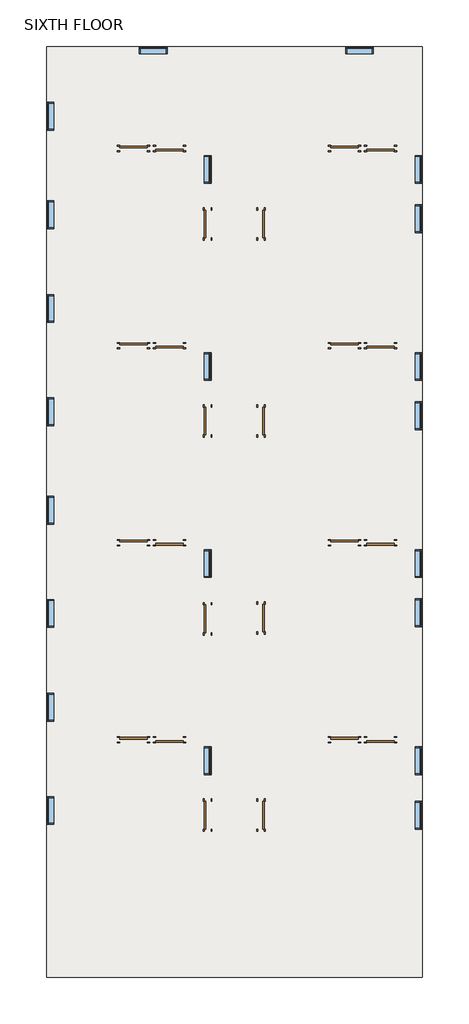
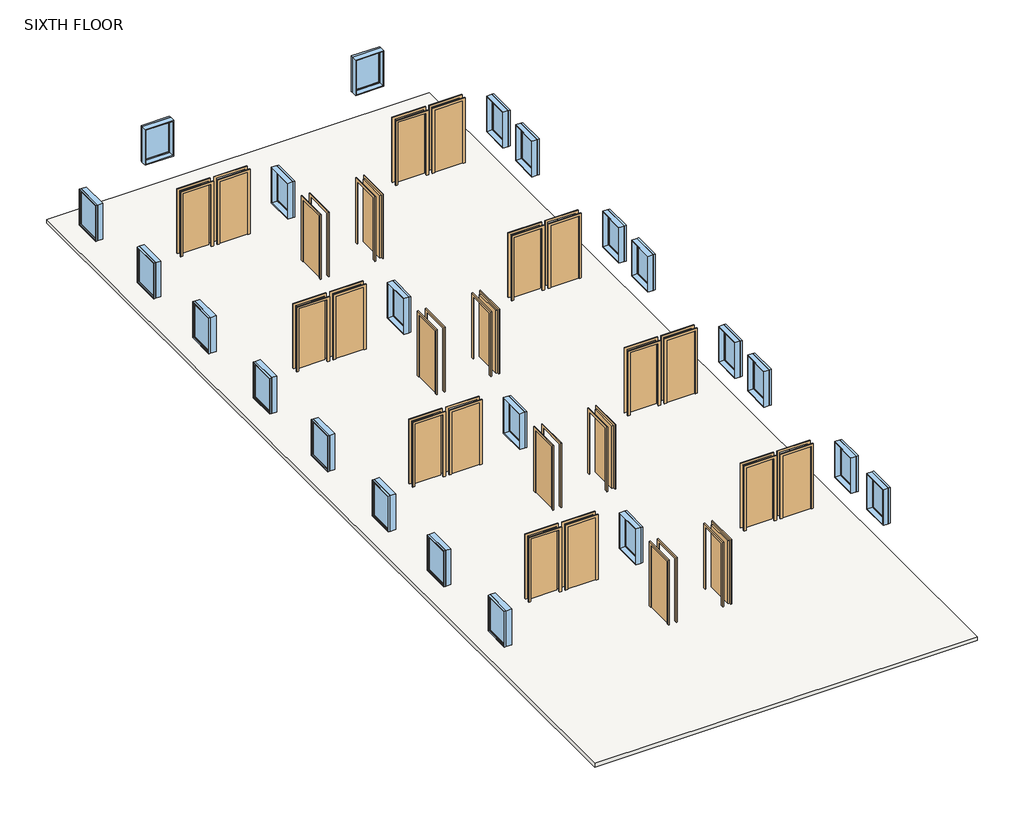
# One storey: 24 doors, 22 windows, 1 slab.
"""IFC4 building model written with IfcOpenShell, lengths in millimetres."""

from ifc_helpers import new_model, si_unit, frame, origin, place, context, project, spatial, polyline, outline, extrude, transform, mapped, element, save
from components import door_686f89d2, door_16372e1c, door_a90ba1ad, door_0ca8825f, window_c1f32544

model = new_model("IFC4")

# Units and contexts
model_context = context("Model", 3, world=origin())
ifc_project = project(units=[si_unit("LENGTHUNIT", "METRE", prefix="MILLI")], contexts=[model_context])

# Site, building, storey
site = spatial("IfcSite", under=ifc_project)
building = spatial("IfcBuilding", under=site)
storey = spatial("IfcBuildingStorey", under=building, Name="SIXTH FLOOR", Elevation=19202.4)

# Doors
placement = place(None, origin())
door_shape = door_686f89d2(model_context)
element("IfcDoor", 1, ObjectType="Single-Flush : 36\" x 84\"", at=placement, inside=storey, context=model_context, shape_type="MappedRepresentation", body=[
    mapped(door_shape, transform((-9863.5902461, 11952.2710592, 19202.4), x_axis=(-1.0, 0.0, 0.0), y_axis=(0.0, -1.0, 0.0), z_axis=(0.0, 0.0, 1.0))),
])
element("IfcDoor", 2, ObjectType="Single-Flush : 36\" x 84\"", at=placement, inside=storey, context=model_context, shape_type="MappedRepresentation", body=[
    mapped(door_shape, transform((-9863.5902461, 5475.2710592, 19202.4), x_axis=(-1.0, 0.0, 0.0), y_axis=(0.0, -1.0, 0.0), z_axis=(0.0, 0.0, 1.0))),
])
element("IfcDoor", 3, ObjectType="Single-Flush : 36\" x 84\"", at=placement, inside=storey, context=model_context, shape_type="MappedRepresentation", body=[
    mapped(door_shape, transform((-9863.5902461, -1001.7289408, 19202.4), x_axis=(-1.0, 0.0, 0.0), y_axis=(0.0, -1.0, 0.0), z_axis=(0.0, 0.0, 1.0))),
])
element("IfcDoor", 4, ObjectType="Single-Flush : 36\" x 84\"", at=placement, inside=storey, context=model_context, shape_type="MappedRepresentation", body=[
    mapped(door_shape, transform((-9863.5902461, -7478.7289408, 19202.4), x_axis=(-1.0, 0.0, 0.0), y_axis=(0.0, -1.0, 0.0), z_axis=(0.0, 0.0, 1.0))),
])
element("IfcDoor", 5, ObjectType="Single-Flush : 36\" x 84\"", at=placement, inside=storey, context=model_context, shape_type="MappedRepresentation", body=[
    mapped(door_shape, transform((-2929.3902461, -7478.7289408, 19202.4), x_axis=(-1.0, 0.0, 0.0), y_axis=(0.0, -1.0, 0.0), z_axis=(0.0, 0.0, 1.0))),
])
element("IfcDoor", 6, ObjectType="Single-Flush : 36\" x 84\"", at=placement, inside=storey, context=model_context, shape_type="MappedRepresentation", body=[
    mapped(door_shape, transform((-2929.3902461, -1001.7289408, 19202.4), x_axis=(-1.0, 0.0, 0.0), y_axis=(0.0, -1.0, 0.0), z_axis=(0.0, 0.0, 1.0))),
])
element("IfcDoor", 7, ObjectType="Single-Flush : 36\" x 84\"", at=placement, inside=storey, context=model_context, shape_type="MappedRepresentation", body=[
    mapped(door_shape, transform((-2929.3902461, 5475.2710592, 19202.4), x_axis=(-1.0, 0.0, 0.0), y_axis=(0.0, -1.0, 0.0), z_axis=(0.0, 0.0, 1.0))),
])
element("IfcDoor", 8, ObjectType="Single-Flush : 36\" x 84\"", at=placement, inside=storey, context=model_context, shape_type="MappedRepresentation", body=[
    mapped(door_shape, transform((-2929.3902461, 11952.2710592, 19202.4), x_axis=(-1.0, 0.0, 0.0), y_axis=(0.0, -1.0, 0.0), z_axis=(0.0, 0.0, 1.0))),
])
door_2_shape = door_16372e1c(model_context)
element("IfcDoor", 9, ObjectType="Single-Flush : 36\" x 84\"", at=placement, inside=storey, context=model_context, shape_type="MappedRepresentation", body=[
    mapped(door_2_shape, transform((-8682.4902461, 11952.2710592, 19202.4), x_axis=(-1.0, 0.0, 0.0), y_axis=(0.0, -1.0, 0.0), z_axis=(0.0, 0.0, 1.0))),
])
element("IfcDoor", 10, ObjectType="Single-Flush : 36\" x 84\"", at=placement, inside=storey, context=model_context, shape_type="MappedRepresentation", body=[
    mapped(door_2_shape, transform((-8682.4902461, 5475.2710592, 19202.4), x_axis=(-1.0, 0.0, 0.0), y_axis=(0.0, -1.0, 0.0), z_axis=(0.0, 0.0, 1.0))),
])
element("IfcDoor", 11, ObjectType="Single-Flush : 36\" x 84\"", at=placement, inside=storey, context=model_context, shape_type="MappedRepresentation", body=[
    mapped(door_2_shape, transform((-8682.4902461, -1001.7289408, 19202.4), x_axis=(-1.0, 0.0, 0.0), y_axis=(0.0, -1.0, 0.0), z_axis=(0.0, 0.0, 1.0))),
])
element("IfcDoor", 12, ObjectType="Single-Flush : 36\" x 84\"", at=placement, inside=storey, context=model_context, shape_type="MappedRepresentation", body=[
    mapped(door_2_shape, transform((-8682.4902461, -7478.7289408, 19202.4), x_axis=(-1.0, 0.0, 0.0), y_axis=(0.0, -1.0, 0.0), z_axis=(0.0, 0.0, 1.0))),
])
element("IfcDoor", 13, ObjectType="Single-Flush : 36\" x 84\"", at=placement, inside=storey, context=model_context, shape_type="MappedRepresentation", body=[
    mapped(door_2_shape, transform((-1748.2902461, -7478.7289408, 19202.4), x_axis=(-1.0, 0.0, 0.0), y_axis=(0.0, -1.0, 0.0), z_axis=(0.0, 0.0, 1.0))),
])
element("IfcDoor", 14, ObjectType="Single-Flush : 36\" x 84\"", at=placement, inside=storey, context=model_context, shape_type="MappedRepresentation", body=[
    mapped(door_2_shape, transform((-1748.2902461, -1001.7289408, 19202.4), x_axis=(-1.0, 0.0, 0.0), y_axis=(0.0, -1.0, 0.0), z_axis=(0.0, 0.0, 1.0))),
])
element("IfcDoor", 15, ObjectType="Single-Flush : 36\" x 84\"", at=placement, inside=storey, context=model_context, shape_type="MappedRepresentation", body=[
    mapped(door_2_shape, transform((-1748.2902461, 5475.2710592, 19202.4), x_axis=(-1.0, 0.0, 0.0), y_axis=(0.0, -1.0, 0.0), z_axis=(0.0, 0.0, 1.0))),
])
element("IfcDoor", 16, ObjectType="Single-Flush : 36\" x 84\"", at=placement, inside=storey, context=model_context, shape_type="MappedRepresentation", body=[
    mapped(door_2_shape, transform((-1748.2902461, 11952.2710592, 19202.4), x_axis=(-1.0, 0.0, 0.0), y_axis=(0.0, -1.0, 0.0), z_axis=(0.0, 0.0, 1.0))),
])
door_3_shape = door_a90ba1ad(model_context)
element("IfcDoor", 17, ObjectType="Single-Flush : 36\" x 84\"", at=placement, inside=storey, context=model_context, shape_type="MappedRepresentation", body=[
    mapped(door_3_shape, transform((-7425.1902461, 9475.7710592, 19202.4), x_axis=(0.0, -1.0, 0.0), y_axis=(1.0, 0.0, 0.0), z_axis=(0.0, 0.0, 1.0))),
])
element("IfcDoor", 18, ObjectType="Single-Flush : 36\" x 84\"", at=placement, inside=storey, context=model_context, shape_type="MappedRepresentation", body=[
    mapped(door_3_shape, transform((-7425.1902461, 2998.7710592, 19202.4), x_axis=(0.0, -1.0, 0.0), y_axis=(1.0, 0.0, 0.0), z_axis=(0.0, 0.0, 1.0))),
])
element("IfcDoor", 19, ObjectType="Single-Flush : 36\" x 84\"", at=placement, inside=storey, context=model_context, shape_type="MappedRepresentation", body=[
    mapped(door_3_shape, transform((-7425.1902461, -3503.6289408, 19202.4), x_axis=(0.0, -1.0, 0.0), y_axis=(1.0, 0.0, 0.0), z_axis=(0.0, 0.0, 1.0))),
])
element("IfcDoor", 20, ObjectType="Single-Flush : 36\" x 84\"", at=placement, inside=storey, context=model_context, shape_type="MappedRepresentation", body=[
    mapped(door_3_shape, transform((-7425.1902461, -9955.2289408, 19202.4), x_axis=(0.0, -1.0, 0.0), y_axis=(1.0, 0.0, 0.0), z_axis=(0.0, 0.0, 1.0))),
])
door_4_shape = door_0ca8825f(model_context)
element("IfcDoor", 21, ObjectType="Single-Flush : 36\" x 84\"", at=placement, inside=storey, context=model_context, shape_type="MappedRepresentation", body=[
    mapped(door_4_shape, transform((-5672.5902461, 9475.7710592, 19202.4), x_axis=(0.0, -1.0, 0.0), y_axis=(1.0, 0.0, 0.0), z_axis=(0.0, 0.0, 1.0))),
])
element("IfcDoor", 22, ObjectType="Single-Flush : 36\" x 84\"", at=placement, inside=storey, context=model_context, shape_type="MappedRepresentation", body=[
    mapped(door_4_shape, transform((-5672.5902461, 2998.7710592, 19202.4), x_axis=(0.0, -1.0, 0.0), y_axis=(1.0, 0.0, 0.0), z_axis=(0.0, 0.0, 1.0))),
])
element("IfcDoor", 23, ObjectType="Single-Flush : 36\" x 84\"", at=placement, inside=storey, context=model_context, shape_type="MappedRepresentation", body=[
    mapped(door_4_shape, transform((-5672.5902461, -3478.2289408, 19202.4), x_axis=(0.0, -1.0, 0.0), y_axis=(1.0, 0.0, 0.0), z_axis=(0.0, 0.0, 1.0))),
])
element("IfcDoor", 24, ObjectType="Single-Flush : 36\" x 84\"", at=placement, inside=storey, context=model_context, shape_type="MappedRepresentation", body=[
    mapped(door_4_shape, transform((-5672.5902461, -9955.2289408, 19202.4), x_axis=(0.0, -1.0, 0.0), y_axis=(1.0, 0.0, 0.0), z_axis=(0.0, 0.0, 1.0))),
])

# Slab
element("IfcSlab", 25, ObjectType="Generic - 12\"", at=placement, inside=storey, context=model_context, shape_type="SweptSolid", body=[
    extrude(outline(polyline([(-376.6902461, 15305.0710592), (-376.6902461, -15289.2289408), (-12721.0902461, -15289.2289408), (-12721.0902461, 15305.0710592), (-376.6902461, 15305.0710592)])), frame((0.0, 0.0, 19075.4), z_axis=(0.0, 0.0, 1.0), x_axis=(1.0, 0.0, 0.0)), (0.0, 0.0, 1.0), 127.0),
])

# Windows
window_shape = window_c1f32544(model_context)
element("IfcWindow", 26, ObjectType="Fixed : 36\" x 48\"", at=placement, inside=storey, context=model_context, shape_type="MappedRepresentation", body=[
    mapped(window_shape, transform((-9177.7902461, 15190.7710592, 19202.4), x_axis=(1.0, 0.0, 0.0), y_axis=(0.0, 1.0, 0.0), z_axis=(0.0, 0.0, 1.0))),
])
element("IfcWindow", 27, ObjectType="Fixed : 36\" x 48\"", at=placement, inside=storey, context=model_context, shape_type="MappedRepresentation", body=[
    mapped(window_shape, transform((-2395.9902461, 15190.7710592, 19202.4), x_axis=(1.0, 0.0, 0.0), y_axis=(0.0, 1.0, 0.0), z_axis=(0.0, 0.0, 1.0))),
])
element("IfcWindow", 28, ObjectType="Fixed : 36\" x 48\"", at=placement, inside=storey, context=model_context, shape_type="MappedRepresentation", body=[
    mapped(window_shape, transform((-490.9902461, 11228.3710592, 19202.4), x_axis=(0.0, -1.0, 0.0), y_axis=(1.0, 0.0, 0.0), z_axis=(0.0, 0.0, 1.0))),
])
element("IfcWindow", 29, ObjectType="Fixed : 36\" x 48\"", at=placement, inside=storey, context=model_context, shape_type="MappedRepresentation", body=[
    mapped(window_shape, transform((-490.9902461, 9609.1210592, 19202.4), x_axis=(0.0, -1.0, 0.0), y_axis=(1.0, 0.0, 0.0), z_axis=(0.0, 0.0, 1.0))),
])
element("IfcWindow", 30, ObjectType="Fixed : 36\" x 48\"", at=placement, inside=storey, context=model_context, shape_type="MappedRepresentation", body=[
    mapped(window_shape, transform((-490.9902461, 4751.3710592, 19202.4), x_axis=(0.0, -1.0, 0.0), y_axis=(1.0, 0.0, 0.0), z_axis=(0.0, 0.0, 1.0))),
])
element("IfcWindow", 31, ObjectType="Fixed : 36\" x 48\"", at=placement, inside=storey, context=model_context, shape_type="MappedRepresentation", body=[
    mapped(window_shape, transform((-490.9902461, 3132.1210592, 19202.4), x_axis=(0.0, -1.0, 0.0), y_axis=(1.0, 0.0, 0.0), z_axis=(0.0, 0.0, 1.0))),
])
element("IfcWindow", 32, ObjectType="Fixed : 36\" x 48\"", at=placement, inside=storey, context=model_context, shape_type="MappedRepresentation", body=[
    mapped(window_shape, transform((-490.9902461, -1725.6289408, 19202.4), x_axis=(0.0, -1.0, 0.0), y_axis=(1.0, 0.0, 0.0), z_axis=(0.0, 0.0, 1.0))),
])
element("IfcWindow", 33, ObjectType="Fixed : 36\" x 48\"", at=placement, inside=storey, context=model_context, shape_type="MappedRepresentation", body=[
    mapped(window_shape, transform((-490.9902461, -3344.8789408, 19202.4), x_axis=(0.0, -1.0, 0.0), y_axis=(1.0, 0.0, 0.0), z_axis=(0.0, 0.0, 1.0))),
])
element("IfcWindow", 34, ObjectType="Fixed : 36\" x 48\"", at=placement, inside=storey, context=model_context, shape_type="MappedRepresentation", body=[
    mapped(window_shape, transform((-490.9902461, -8202.6289408, 19202.4), x_axis=(0.0, -1.0, 0.0), y_axis=(1.0, 0.0, 0.0), z_axis=(0.0, 0.0, 1.0))),
])
element("IfcWindow", 35, ObjectType="Fixed : 36\" x 48\"", at=placement, inside=storey, context=model_context, shape_type="MappedRepresentation", body=[
    mapped(window_shape, transform((-490.9902461, -9993.3289408, 19202.4), x_axis=(0.0, -1.0, 0.0), y_axis=(1.0, 0.0, 0.0), z_axis=(0.0, 0.0, 1.0))),
])
element("IfcWindow", 36, ObjectType="Fixed : 36\" x 48\"", at=placement, inside=storey, context=model_context, shape_type="MappedRepresentation", body=[
    mapped(window_shape, transform((-12606.7902461, -9764.7289408, 19202.4), x_axis=(0.0, 1.0, 0.0), y_axis=(-1.0, 0.0, 0.0), z_axis=(0.0, 0.0, 1.0))),
])
element("IfcWindow", 37, ObjectType="Fixed : 36\" x 48\"", at=placement, inside=storey, context=model_context, shape_type="MappedRepresentation", body=[
    mapped(window_shape, transform((-12606.7902461, -6373.8289408, 19202.4), x_axis=(0.0, 1.0, 0.0), y_axis=(-1.0, 0.0, 0.0), z_axis=(0.0, 0.0, 1.0))),
])
element("IfcWindow", 38, ObjectType="Fixed : 36\" x 48\"", at=placement, inside=storey, context=model_context, shape_type="MappedRepresentation", body=[
    mapped(window_shape, transform((-12606.7902461, -3287.7289408, 19202.4), x_axis=(0.0, 1.0, 0.0), y_axis=(-1.0, 0.0, 0.0), z_axis=(0.0, 0.0, 1.0))),
])
element("IfcWindow", 39, ObjectType="Fixed : 36\" x 48\"", at=placement, inside=storey, context=model_context, shape_type="MappedRepresentation", body=[
    mapped(window_shape, transform((-12606.7902461, 103.1710592, 19202.4), x_axis=(0.0, 1.0, 0.0), y_axis=(-1.0, 0.0, 0.0), z_axis=(0.0, 0.0, 1.0))),
])
element("IfcWindow", 40, ObjectType="Fixed : 36\" x 48\"", at=placement, inside=storey, context=model_context, shape_type="MappedRepresentation", body=[
    mapped(window_shape, transform((-12606.7902461, 3341.6710592, 19202.4), x_axis=(0.0, 1.0, 0.0), y_axis=(-1.0, 0.0, 0.0), z_axis=(0.0, 0.0, 1.0))),
])
element("IfcWindow", 41, ObjectType="Fixed : 36\" x 48\"", at=placement, inside=storey, context=model_context, shape_type="MappedRepresentation", body=[
    mapped(window_shape, transform((-12606.7902461, 6732.5710592, 19202.4), x_axis=(0.0, 1.0, 0.0), y_axis=(-1.0, 0.0, 0.0), z_axis=(0.0, 0.0, 1.0))),
])
element("IfcWindow", 42, ObjectType="Fixed : 36\" x 48\"", at=placement, inside=storey, context=model_context, shape_type="MappedRepresentation", body=[
    mapped(window_shape, transform((-12606.7902461, 9818.6710592, 19202.4), x_axis=(0.0, 1.0, 0.0), y_axis=(-1.0, 0.0, 0.0), z_axis=(0.0, 0.0, 1.0))),
])
element("IfcWindow", 43, ObjectType="Fixed : 36\" x 48\"", at=placement, inside=storey, context=model_context, shape_type="MappedRepresentation", body=[
    mapped(window_shape, transform((-12606.7902461, 13057.1710592, 19202.4), x_axis=(0.0, 1.0, 0.0), y_axis=(-1.0, 0.0, 0.0), z_axis=(0.0, 0.0, 1.0))),
])
element("IfcWindow", 44, ObjectType="Fixed : 36\" x 48\"", at=placement, inside=storey, context=model_context, shape_type="MappedRepresentation", body=[
    mapped(window_shape, transform((-7425.1902461, 11228.3710592, 19202.4), x_axis=(0.0, -1.0, 0.0), y_axis=(1.0, 0.0, 0.0), z_axis=(0.0, 0.0, 1.0))),
])
element("IfcWindow", 45, ObjectType="Fixed : 36\" x 48\"", at=placement, inside=storey, context=model_context, shape_type="MappedRepresentation", body=[
    mapped(window_shape, transform((-7425.1902461, 4751.3710592, 19202.4), x_axis=(0.0, -1.0, 0.0), y_axis=(1.0, 0.0, 0.0), z_axis=(0.0, 0.0, 1.0))),
])
element("IfcWindow", 46, ObjectType="Fixed : 36\" x 48\"", at=placement, inside=storey, context=model_context, shape_type="MappedRepresentation", body=[
    mapped(window_shape, transform((-7425.1902461, -1725.6289408, 19202.4), x_axis=(0.0, -1.0, 0.0), y_axis=(1.0, 0.0, 0.0), z_axis=(0.0, 0.0, 1.0))),
])
element("IfcWindow", 47, ObjectType="Fixed : 36\" x 48\"", at=placement, inside=storey, context=model_context, shape_type="MappedRepresentation", body=[
    mapped(window_shape, transform((-7425.1902461, -8202.6289408, 19202.4), x_axis=(0.0, -1.0, 0.0), y_axis=(1.0, 0.0, 0.0), z_axis=(0.0, 0.0, 1.0))),
])

save(model, "model.ifc")

# Revit data of these elements
# Type "Single-Flush : 36\" x 84\""
#   Type Mark = "1"
#   Construction Type Id = "MDOOR"
#   Assembly Code = "C1020"
#   Analytic Construction = "Metal"
#   Thickness = 0' - 2"
#   Heat Transfer Coefficient (U) = 0.651978 BTU/(h·ft²·°F)
#   Height = 7' - 0"
#   Trim Projection Ext = 0' - 1"
#   Trim Projection Int = 0' - 1"
#   Trim Width = 0' - 3"
#   Width = 3' - 0"
#   Define Thermal Properties by = 1
#   Door Material = Door - Panel
#   Frame Material = Door - Frame
#   Visual Light Transmittance = 0
#   Solar Heat Gain Coefficient = 0
#   Function = (empty or 0)
#   Wall Closure = (empty or 0)
# Type "Generic - 12\""
#   Assembly Code = "B1010"
#   Function = 0
#   Layers, outside or top first: 0' - 5" no material (function 1)
# Type "Fixed : 36\" x 48\""
#   Type Mark = "1"
#   Construction Type Id = "GSP4R"
#   Assembly Code = "B2020100"
#   Analytic Construction = "1/8 in Pilkington single glazing"
#   Visual Light Transmittance = 0.9
#   Solar Heat Gain Coefficient = 0.78
#   Heat Transfer Coefficient (U) = 0.6496 BTU/(h·ft²·°F)
#   Height = 4' - 0"
#   Default Sill Height = 3' - 0"
#   Width = 3' - 0"
#   Window Inset = 0' - 0 3/4"
#   Define Thermal Properties by = 1
#   Glass Pane Material = Glass
#   Sash Material = Sash
#   Wall Closure = (empty or 0)
# Elements 1, 2, 3, 4, 5, 6, 7, 8, 9, 10, 11, 12, 13, 14, 15, 16, 17, 18, 19, 20, 21, 22, 23, 24 (IfcDoor, "Single-Flush : 36\" x 84\"")
#   Phase Created = New Construction
#   Materials on its faces: "Door - Frame", "Door - Panel"
# Element 25 (IfcSlab, "Generic - 12\"")
#   Height Offset From Level = 0' - 0"
#   Phase Created = New Construction
#   Materials on its faces: "Default Floor"
# Element 26 (IfcWindow, "Fixed : 36\" x 48\"")
#   Mark = "139"
#   Phase Created = New Construction
#   Materials on its faces: "Sash", "Glass"
# Element 27 (IfcWindow, "Fixed : 36\" x 48\"")
#   Mark = "140"
#   Phase Created = New Construction
#   Materials on its faces: "Sash", "Glass"
# Element 28 (IfcWindow, "Fixed : 36\" x 48\"")
#   Mark = "141"
#   Phase Created = New Construction
#   Materials on its faces: "Sash", "Glass"
# Element 29 (IfcWindow, "Fixed : 36\" x 48\"")
#   Mark = "142"
#   Phase Created = New Construction
#   Materials on its faces: "Sash", "Glass"
# Element 30 (IfcWindow, "Fixed : 36\" x 48\"")
#   Mark = "143"
#   Phase Created = New Construction
#   Materials on its faces: "Sash", "Glass"
# Element 31 (IfcWindow, "Fixed : 36\" x 48\"")
#   Mark = "144"
#   Phase Created = New Construction
#   Materials on its faces: "Sash", "Glass"
# Element 32 (IfcWindow, "Fixed : 36\" x 48\"")
#   Mark = "145"
#   Phase Created = New Construction
#   Materials on its faces: "Sash", "Glass"
# Element 33 (IfcWindow, "Fixed : 36\" x 48\"")
#   Mark = "146"
#   Phase Created = New Construction
#   Materials on its faces: "Sash", "Glass"
# Element 34 (IfcWindow, "Fixed : 36\" x 48\"")
#   Mark = "147"
#   Phase Created = New Construction
#   Materials on its faces: "Sash", "Glass"
# Element 35 (IfcWindow, "Fixed : 36\" x 48\"")
#   Mark = "148"
#   Phase Created = New Construction
#   Materials on its faces: "Sash", "Glass"
# Element 36 (IfcWindow, "Fixed : 36\" x 48\"")
#   Mark = "149"
#   Phase Created = New Construction
#   Materials on its faces: "Sash", "Glass"
# Element 37 (IfcWindow, "Fixed : 36\" x 48\"")
#   Mark = "150"
#   Phase Created = New Construction
#   Materials on its faces: "Sash", "Glass"
# Element 38 (IfcWindow, "Fixed : 36\" x 48\"")
#   Mark = "151"
#   Phase Created = New Construction
#   Materials on its faces: "Sash", "Glass"
# Element 39 (IfcWindow, "Fixed : 36\" x 48\"")
#   Mark = "152"
#   Phase Created = New Construction
#   Materials on its faces: "Sash", "Glass"
# Element 40 (IfcWindow, "Fixed : 36\" x 48\"")
#   Mark = "153"
#   Phase Created = New Construction
#   Materials on its faces: "Sash", "Glass"
# Element 41 (IfcWindow, "Fixed : 36\" x 48\"")
#   Mark = "154"
#   Phase Created = New Construction
#   Materials on its faces: "Sash", "Glass"
# Element 42 (IfcWindow, "Fixed : 36\" x 48\"")
#   Mark = "155"
#   Phase Created = New Construction
#   Materials on its faces: "Sash", "Glass"
# Element 43 (IfcWindow, "Fixed : 36\" x 48\"")
#   Mark = "156"
#   Phase Created = New Construction
#   Materials on its faces: "Sash", "Glass"
# Element 44 (IfcWindow, "Fixed : 36\" x 48\"")
#   Mark = "157"
#   Phase Created = New Construction
#   Materials on its faces: "Sash", "Glass"
# Element 45 (IfcWindow, "Fixed : 36\" x 48\"")
#   Mark = "158"
#   Phase Created = New Construction
#   Materials on its faces: "Sash", "Glass"
# Element 46 (IfcWindow, "Fixed : 36\" x 48\"")
#   Mark = "159"
#   Phase Created = New Construction
#   Materials on its faces: "Sash", "Glass"
# Element 47 (IfcWindow, "Fixed : 36\" x 48\"")
#   Mark = "160"
#   Phase Created = New Construction
#   Materials on its faces: "Sash", "Glass"
# Materials
#   "Door - Panel": class "Wood", colour RGB 210 159 95, transparency 0
#   "Door - Frame": colour RGB 118 70 51, transparency 0
#   "Glass": class "Glass", colour RGB 0 128 192, transparency 0.75, Description = "Soda Lime Glass", Cost = 0
#   "Sash": class "Wood", colour RGB 224 178 126, transparency 0
#   "Default Floor": colour RGB 128 128 128, transparency 0
